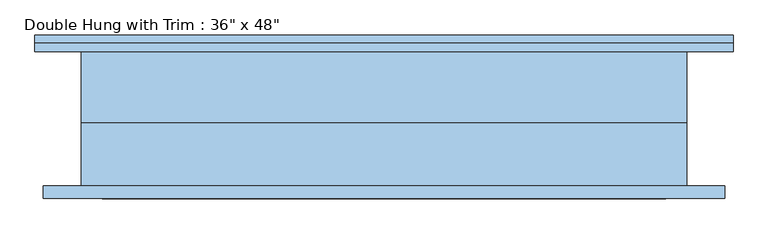
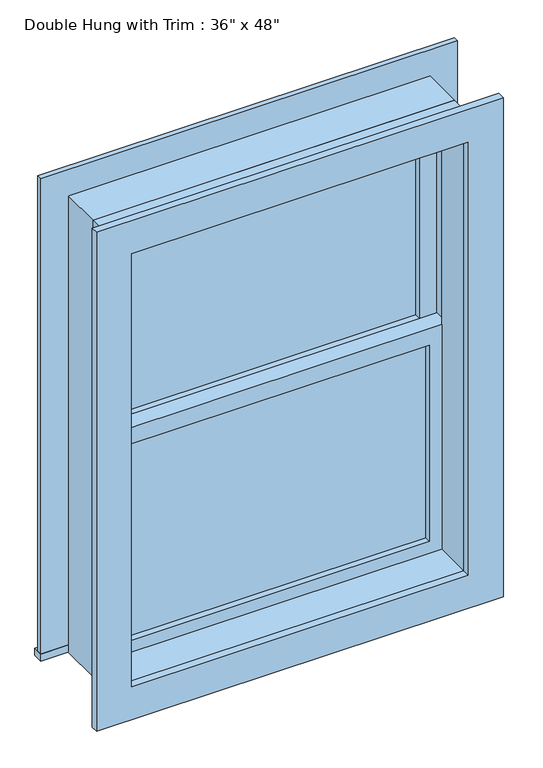
"""IFC4 building model written with IfcOpenShell, lengths in millimetres: window geometry."""

from ifc_helpers import new_model, si_unit, frame, origin, place, context, project, spatial, polyline, outline, extrude, source, transform, mapped, element, save


def window_31198920(model_context):
    return source(origin(), model_context, "Body", "SweptSolid", [
        extrude(outline(polyline([(-393.7, 22.225), (393.7, 22.225), (393.7, 9.525), (-393.7, 9.525), (-393.7, 22.225)])), frame((0.0, 0.0, 977.9), z_axis=(0.0, 0.0, 1.0), x_axis=(1.0, 0.0, 0.0)), (0.0, 0.0, 1.0), 523.875),
        extrude(outline(polyline([(1546.225, -438.15), (933.45, -438.15), (933.45, 438.15), (1546.225, 438.15), (1546.225, -438.15)]), holes=[polyline([(1501.775, -393.7), (1501.775, 393.7), (977.9, 393.7), (977.9, -393.7), (1501.775, -393.7)])]), frame((0.0, -6.35, 0.0), z_axis=(0.0, 1.0, 0.0), x_axis=(0.0, 0.0, 1.0)), (0.0, 0.0, 1.0), 44.45),
        extrude(outline(polyline([(-527.05, 127.0), (527.05, 127.0), (527.05, 101.6), (-527.05, 101.6), (-527.05, 127.0)])), frame((0.0, 0.0, 914.4), z_axis=(0.0, 0.0, 1.0), x_axis=(1.0, 0.0, 0.0)), (0.0, 0.0, 1.0), 19.05),
        extrude(outline(polyline([(2114.55, -438.15), (2114.55, 438.15), (933.45, 438.15), (933.45, 527.05), (2203.45, 527.05), (2203.45, -527.05), (933.45, -527.05), (933.45, -438.15), (2114.55, -438.15)])), frame((0.0, 101.6, 0.0), z_axis=(0.0, 1.0, 0.0), x_axis=(0.0, 0.0, 1.0)), (0.0, 0.0, 1.0), 12.7),
        extrude(outline(polyline([(2190.75, 514.35), (2190.75, -514.35), (857.25, -514.35), (857.25, 514.35), (2190.75, 514.35)]), holes=[polyline([(2101.85, 425.45), (946.15, 425.45), (946.15, -425.45), (2101.85, -425.45), (2101.85, 425.45)])]), frame((0.0, -120.65, 0.0), z_axis=(0.0, 1.0, 0.0), x_axis=(0.0, 0.0, 1.0)), (0.0, 0.0, 1.0), 19.05),
        extrude(outline(polyline([(393.7, 53.975), (-393.7, 53.975), (-393.7, 66.675), (393.7, 66.675), (393.7, 53.975)])), frame((0.0, 0.0, 1546.225), z_axis=(0.0, 0.0, 1.0), x_axis=(1.0, 0.0, 0.0)), (0.0, 0.0, 1.0), 523.875),
        extrude(outline(polyline([(2114.55, -438.15), (1501.775, -438.15), (1501.775, 438.15), (2114.55, 438.15), (2114.55, -438.15)]), holes=[polyline([(2070.1, -393.7), (2070.1, 393.7), (1546.225, 393.7), (1546.225, -393.7), (2070.1, -393.7)])]), frame((0.0, 38.1, 0.0), z_axis=(0.0, 1.0, 0.0), x_axis=(0.0, 0.0, 1.0)), (0.0, 0.0, 1.0), 44.45),
        extrude(outline(polyline([(2133.6, -457.2), (914.4, -457.2), (914.4, 457.2), (2133.6, 457.2), (2133.6, -457.2)]), holes=[polyline([(2101.85, -425.45), (2101.85, 425.45), (946.15, 425.45), (946.15, -425.45), (2101.85, -425.45)])]), frame((0.0, -101.6, 0.0), z_axis=(0.0, 1.0, 0.0), x_axis=(0.0, 0.0, 1.0)), (0.0, 0.0, 1.0), 95.25),
        extrude(outline(polyline([(2133.6, 457.2), (2133.6, -457.2), (914.4, -457.2), (914.4, 457.2), (2133.6, 457.2)]), holes=[polyline([(2114.55, 438.15), (933.45, 438.15), (933.45, -438.15), (2114.55, -438.15), (2114.55, 438.15)])]), frame((0.0, -6.35, 0.0), z_axis=(0.0, 1.0, 0.0), x_axis=(0.0, 0.0, 1.0)), (0.0, 0.0, 1.0), 107.95),
    ])


if __name__ == "__main__":
    model = new_model("IFC4")
    model_context = context("Model", 3, world=origin())
    ifc_project = project(units=[si_unit("LENGTHUNIT", "METRE", prefix="MILLI")], contexts=[model_context])
    site = spatial("IfcSite", under=ifc_project)
    building = spatial("IfcBuilding", under=site)
    placement = place(None, origin())
    window_shape = window_31198920(model_context)
    element("IfcWindow", 1, ObjectType="Double Hung with Trim : 36\" x 48\"", at=placement, inside=building, context=model_context, shape_type="MappedRepresentation", body=[
        mapped(window_shape, transform((0.0, 0.0, 0.0), x_axis=(1.0, 0.0, 0.0), y_axis=(0.0, 1.0, 0.0), z_axis=(0.0, 0.0, 1.0))),
    ])
    save(model, "model.ifc")

# Revit data of these elements
# Type "Double Hung with Trim : 36\" x 48\""
#   Type Mark = "15"
#   Construction Type Id = "GSP4R"
#   Assembly Code = "B2020100"
#   Analytic Construction = "1/8 in Pilkington single glazing"
#   Visual Light Transmittance = 0.9
#   Solar Heat Gain Coefficient = 0.78
#   Heat Transfer Coefficient (U) = 0.6496 BTU/(h·ft²·°F)
#   Height = 4' - 0"
#   Default Sill Height = 3' - 0"
#   Trim Projection - Ext. = 0' - 0 1/2"
#   Trim Projection - Int. = 0' - 0 3/4"
#   Trim Width - Exterior = 0' - 3 1/2"
#   Trim Width - Interior = 0' - 3 1/2"
#   Width = 3' - 0"
#   Window Inset = 0' - 0 3/4"
#   Define Thermal Properties by = 1
#   Glass Pane Material = Glass
#   Sash Material = Structure, Steel Bar Joist Layer
#   Trim Exterior Material = Vapor Retarder
#   Trim Interior Material = Vapor Retarder
#   Wall Closure = (empty or 0)
# Element 1 (IfcWindow, "Double Hung with Trim : 36\" x 48\"")
#   Materials on its faces: "Structure, Steel Bar Joist Layer", "Vapor Retarder", "Glass"
# Materials
#   "Glass": class "Glass", colour RGB 0 128 192, transparency 0.75, Description = "Soda Lime Glass", Cost = 0
#   "Structure, Steel Bar Joist Layer": class "Metal", colour RGB 127 127 127, transparency 0, Description = "Bar joists, thermal airspace", Cost = 0
#   "Vapor Retarder": class "Generic", colour RGB 127 127 127, transparency 0, Description = "Polyethylene film membrane", Cost = 0
